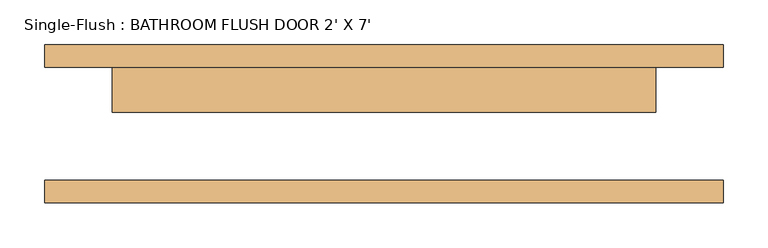
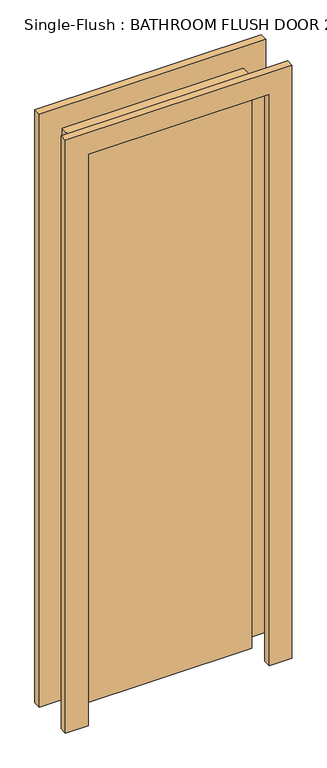
"""IFC4 building model written with IfcOpenShell, lengths in millimetres: door geometry, Single-Flush : BATHROOM FLUSH DOOR 2' X 7'."""

from ifc_helpers import new_model, si_unit, frame, origin, origin_with_axes, place, context, project, spatial, polyline, outline, extrude, source, transform, mapped, element, save


def single_flush_bathroom_flush_door_2_x_7_025d1c86(model_context):
    return source(origin(), model_context, "Body", "SweptSolid", [
        extrude(outline(polyline([(2108.2, -381.0), (0.0, -381.0), (0.0, -304.8), (2032.0, -304.8), (2032.0, 304.8), (0.0, 304.8), (0.0, 381.0), (2108.2, 381.0), (2108.2, -381.0)])), frame((0.0, 63.5, 0.0), z_axis=(0.0, 1.0, 0.0), x_axis=(0.0, 0.0, 1.0)), (0.0, 0.0, 1.0), 25.4),
        extrude(outline(polyline([(2108.2, 381.0), (2108.2, -381.0), (0.0, -381.0), (0.0, -304.8), (2032.0, -304.8), (2032.0, 304.8), (0.0, 304.8), (0.0, 381.0), (2108.2, 381.0)])), frame((0.0, -88.9, 0.0), z_axis=(0.0, 1.0, 0.0), x_axis=(0.0, 0.0, 1.0)), (0.0, 0.0, 1.0), 25.4),
        extrude(outline(polyline([(304.8, 12.7), (-304.8, 12.7), (-304.8, 63.5), (304.8, 63.5), (304.8, 12.7)])), origin_with_axes(), (0.0, 0.0, 1.0), 2032.0),
    ])


if __name__ == "__main__":
    model = new_model("IFC4")
    model_context = context("Model", 3, world=origin())
    ifc_project = project(units=[si_unit("LENGTHUNIT", "METRE", prefix="MILLI")], contexts=[model_context])
    site = spatial("IfcSite", under=ifc_project)
    building = spatial("IfcBuilding", under=site)
    placement = place(None, origin())
    single_flush_bathroom_flush_door_2_x_7_shape = single_flush_bathroom_flush_door_2_x_7_025d1c86(model_context)
    element("IfcDoor", 1, ObjectType="Single-Flush : BATHROOM FLUSH DOOR 2' X 7'", at=placement, inside=building, context=model_context, shape_type="MappedRepresentation", body=[
        mapped(single_flush_bathroom_flush_door_2_x_7_shape, transform((0.0, 0.0, 0.0), x_axis=(1.0, 0.0, 0.0), y_axis=(0.0, 1.0, 0.0), z_axis=(0.0, 0.0, 1.0))),
    ])
    save(model, "model.ifc")

# Revit data of these elements
# Type "Single-Flush : BATHROOM FLUSH DOOR 2' X 7'"
#   Type Mark = "8"
#   Construction Type Id = "MDOOR"
#   Assembly Code = "C1020"
#   Analytic Construction = "Metal"
#   Thickness = 0' - 2"
#   Heat Transfer Coefficient (U) = 0.651978 BTU/(h·ft²·°F)
#   Height = 6' - 8"
#   Trim Projection Ext = 0' - 1"
#   Trim Projection Int = 0' - 1"
#   Trim Width = 0' - 3"
#   Width = 2' - 0"
#   Define Thermal Properties by = 1
#   Door Material = Door - Panel
#   Frame Material = Door - Frame
#   Visual Light Transmittance = 0
#   Solar Heat Gain Coefficient = 0
#   Function = (empty or 0)
#   Wall Closure = (empty or 0)
# Element 1 (IfcDoor, "Single-Flush : BATHROOM FLUSH DOOR 2' X 7'")
#   Materials on its faces: "Door - Frame", "Door - Panel"
# Materials
#   "Door - Panel": class "Wood", colour RGB 210 159 95, transparency 0, Cost = 0
#   "Door - Frame": colour RGB 118 70 51, transparency 0, Cost = 0
